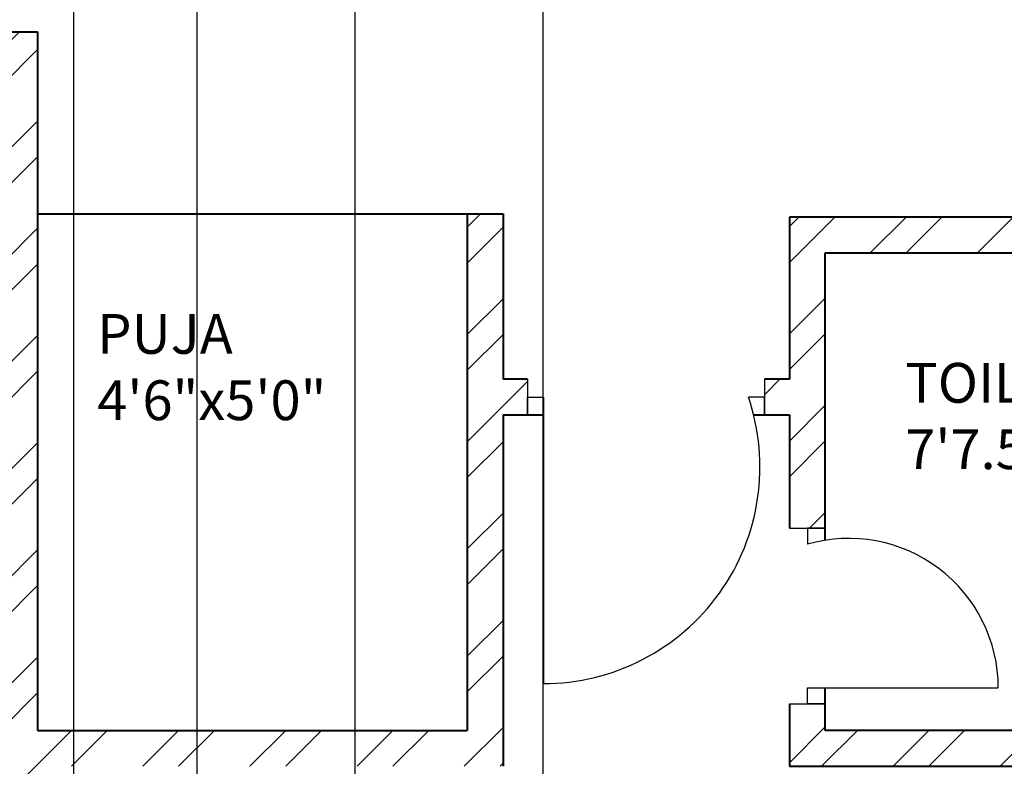
# Model space of a CAD drawing. Units: inches. Extents: x 1601 to 2297, y 1496 to 2631.
# Tile 24 of 57: x 2033 to 2157, y 1793 to 1887. Entities that reach past the tile are written whole.
import ezdxf

# ---------------------------------------------------------------- set-up
doc = ezdxf.new("R2010")
doc.units = ezdxf.units.IN
for name, color, linetype, lineweight in [('A-ANNO-DIMS', 2, 'Continuous', 18), ('A-AREA-IDEN', 7, 'Continuous', 18), ('A-DOOR', 21, 'Continuous', 25), ('A-WALL', 7, 'Continuous', 40), ('A-WALL-PATT', 215, 'Continuous', 13)]:
    doc.layers.add(name, color=color, linetype=linetype, lineweight=lineweight)
doc.styles.get("Standard").update_dxf_attribs({"font": 'arial.ttf'})
doc.dimstyles.get("Standard").update_dxf_attribs({"dimtxt": 0.18, "dimasz": 0.18, "dimexe": 0.18, "dimexo": 0.0625, "dimgap": 0.09, "dimtad": 0, "dimtih": 1, "dimtoh": 1, "dimdec": 4, "dimzin": 0, "dimdsep": 46, "dimtxsty": 'Standard', "dimcen": 0.09, "dimadec": 0, "dimazin": 0, "dimtfac": 1, "dimtdec": 4, "dimtofl": 0, "dimtmove": 0, "dimatfit": 3, "dimfxl": 1, "dimtolj": 1, "dimtzin": 0, "dimarcsym": 0})

# ---------------------------------------------------------------- blocks, each defined once
blk = doc.blocks.new('*D39')
at = {"layer": 'A-ANNO-DIMS', "color": 0, "lineweight": -2, "transparency": 16777216}
for p, q in [((2055.55, 1981.76), (2055.55, 1513.75)), ((2099.05, 1981.76), (2099.05, 1513.75)), ((2055.73, 1513.93), (2076.97, 1513.93)), ((2098.87, 1513.93), (2077.63, 1513.93))]:
    blk.add_line(p, q, dxfattribs=at)
at = {"layer": 'A-ANNO-DIMS', "color": 0, "transparency": 16777216}
for points in [[(2055.73, 1513.96), (2055.73, 1513.9), (2055.55, 1513.93)], [(2098.87, 1513.96), (2098.87, 1513.9), (2099.05, 1513.93)]]:
    blk.add_solid(points, dxfattribs=at)
at = {"layer": 'Defpoints', "color": 0, "transparency": 16777216}
for p in [(2055.55, 1981.83), (2099.05, 1981.83), (2099.05, 1513.93)]:
    blk.add_point(p, dxfattribs=at)
at = {"layer": 'A-ANNO-DIMS', "color": 0, "transparency": 16777216, "insert": (2077.3, 1513.93), "char_height": 0.18, "attachment_point": 5}
blk.add_mtext('\\A1;43.5', dxfattribs=at)
blk = doc.blocks.new('*D41')
at = {"layer": 'A-ANNO-DIMS', "color": 0, "lineweight": -2, "transparency": 16777216}
for p, q in [((2075.4, 2070.14), (2075.4, 1513.75)), ((2040.04, 2066.51), (2040.04, 1513.75)), ((2040.22, 1513.93), (2057.32, 1513.93)), ((2075.22, 1513.93), (2058.11, 1513.93))]:
    blk.add_line(p, q, dxfattribs=at)
at = {"layer": 'A-ANNO-DIMS', "color": 0, "transparency": 16777216}
for points in [[(2040.22, 1513.96), (2040.22, 1513.9), (2040.04, 1513.93)], [(2075.22, 1513.96), (2075.22, 1513.9), (2075.4, 1513.93)]]:
    blk.add_solid(points, dxfattribs=at)
at = {"layer": 'Defpoints', "color": 0, "transparency": 16777216}
for p in [(2075.4, 2070.2), (2040.04, 2066.58), (2075.4, 1513.93)]:
    blk.add_point(p, dxfattribs=at)
at = {"layer": 'A-ANNO-DIMS', "color": 0, "transparency": 16777216, "insert": (2057.72, 1513.93), "char_height": 0.18, "attachment_point": 5}
blk.add_mtext('\\A1;35.36', dxfattribs=at)

msp = doc.modelspace()

# ---------------------------------------------------------------- hatches: boundary and pattern name
at = {"layer": 'A-WALL-PATT'}
h = msp.add_hatch(dxfattribs=at)
h.set_pattern_fill('ANSI32', color=256)
h.paths.add_polyline_path([(1842.0336, 2528.0767), (1842.0336, 2532.3254), (1686.0373, 2532.3254), (1686.0373, 2492.9493), (1695.0373, 2492.9493), (1695.0373, 2523.3254), (1827.0373, 2523.3254), (1827.0373, 2416.8254), (1834.6225, 2416.8254), (1834.6225, 2419.0754), (1834.6225, 2421.3254), (1831.5373, 2421.3254), (1831.5373, 2523.3254), (1842.0336, 2523.3254)])
h.paths.add_polyline_path([(1695.0373, 2432.9493), (1686.0373, 2432.9493), (1686.0373, 2325.989), (1695.0373, 2325.989), (1695.0373, 2347.8254), (1827.0373, 2347.8254), (1827.0373, 2287.8254), (1823.2991, 2287.8254), (1823.2991, 2283.3254), (1847.9422, 2283.3254), (1847.9422, 2285.5754), (1847.9422, 2287.8254), (1831.5373, 2287.8254), (1831.5373, 2347.8254), (1846.9946, 2347.8254), (1846.9946, 2350.0754), (1846.9946, 2352.3254), (1695.0373, 2352.3254)])
h.paths.add_polyline_path([(1807.1169, 1573.5395), (2055.0405, 1573.5395), (2055.0405, 1610.6322), (1807.1169, 1610.6322)], flags=9)
h.paths.add_polyline_path([(1841.1631, 1712.7967), (1870.3957, 1712.7967), (1870.3957, 1731.454), (1841.1631, 1731.454)], flags=9)
h.paths.add_polyline_path([(2144.3862, 1772.185), (2191.0233, 1772.185), (2191.0233, 1790.8423), (2144.3862, 1790.8423)], flags=9)
h.paths.add_polyline_path([(2143.0128, 1827.3312), (2177.9958, 1827.3312), (2177.9958, 1845.9886), (2143.0128, 1845.9886)], flags=9)
h.paths.add_polyline_path([(2041.2439, 1833.5691), (2070.8516, 1833.5691), (2070.8516, 1852.2264), (2041.2439, 1852.2264)], flags=9)
h.paths.add_polyline_path([(2097.2791, 1947.0598), (2134.2061, 1947.0598), (2134.2061, 1965.7171), (2097.2791, 1965.7171)], flags=9)
h.paths.add_polyline_path([(2214.995, 1904.3124), (2214.995, 1942.2899), (2196.3376, 1942.2899), (2196.3376, 1904.3124)], flags=9)
h.paths.add_polyline_path([(2186.6284, 2043.8031), (2219.7935, 2043.8031), (2219.7935, 2062.4605), (2186.6284, 2062.4605)], flags=9)
h.paths.add_polyline_path([(2064.0877, 2031.616), (2097.4949, 2031.616), (2097.4949, 2050.2734), (2064.0877, 2050.2734)], flags=9)
h.paths.add_polyline_path([(1973.1349, 1986.0688), (2008.4009, 1986.0688), (2008.4009, 2004.7261), (1973.1349, 2004.7261)], flags=9)
h.paths.add_polyline_path([(1976.3676, 2106.9635), (2005.7469, 2106.9635), (2005.7469, 2125.6209), (1976.3676, 2125.6209)], flags=9)
h.paths.add_polyline_path([(1991.7852, 2180.4863), (2027.0513, 2180.4863), (2027.0513, 2199.1437), (1991.7852, 2199.1437)], flags=9)
h.paths.add_polyline_path([(2106.1801, 2187.9359), (2152.2101, 2187.9359), (2152.2101, 2206.5932), (2106.1801, 2206.5932)], flags=9)
h.paths.add_polyline_path([(2148.6686, 2262.2542), (2182.318, 2262.2542), (2182.318, 2280.9115), (2148.6686, 2280.9115)], flags=9)
h.paths.add_polyline_path([(2041.6327, 2252.8147), (2071.2405, 2252.8147), (2071.2405, 2271.4721), (2041.6327, 2271.4721)], flags=9)
h.paths.add_polyline_path([(2063.9734, 2375.4265), (2100.9004, 2375.4265), (2100.9004, 2394.0839), (2063.9734, 2394.0839)], flags=9)
h.paths.add_polyline_path([(2216.4955, 2330.9748), (2216.4955, 2370.2654), (2197.8381, 2370.2654), (2197.8381, 2330.9748)], flags=9)
h.paths.add_polyline_path([(2179.1416, 2485.8687), (2212.3067, 2485.8687), (2212.3067, 2504.5261), (2179.1416, 2504.5261)], flags=9)
h.paths.add_polyline_path([(2078.7442, 2471.1516), (2112.1514, 2471.1516), (2112.1514, 2489.809), (2078.7442, 2489.809)], flags=9)
h.paths.add_polyline_path([(1915.9631, 2329.4668), (1952.8902, 2329.4668), (1952.8902, 2348.1241), (1915.9631, 2348.1241)], flags=9)
h.paths.add_polyline_path([(1904.3189, 2499.6709), (1940.4512, 2499.6709), (1940.4512, 2518.3282), (1904.3189, 2518.3282)], flags=9)
h.paths.add_polyline_path([(1892.3665, 2100.4595), (1925.6374, 2100.4595), (1925.6374, 2119.1169), (1892.3665, 2119.1169)], flags=9)
h.paths.add_polyline_path([(1909.2984, 1805.9631), (1946.2254, 1805.9631), (1946.2254, 1824.6205), (1909.2984, 1824.6205)], flags=9)
h.paths.add_polyline_path([(1934.6056, 1658.616), (1970.738, 1658.616), (1970.738, 1677.2733), (1934.6056, 1677.2733)], flags=9)
h.paths.add_polyline_path([(1711.2052, 1789.8902), (1750.0456, 1789.8902), (1750.0456, 1808.5476), (1711.2052, 1808.5476)], flags=9)
h.paths.add_polyline_path([(1742.7874, 1854.6743), (1771.9449, 1854.6743), (1771.9449, 1873.3317), (1742.7874, 1873.3317)], flags=9)
h.paths.add_polyline_path([(1807.3592, 1997.7912), (1850.1116, 1997.7912), (1850.1116, 2016.4486), (1807.3592, 2016.4486)], flags=9)
h.paths.add_polyline_path([(1717.4579, 2237.7844), (1760.2103, 2237.7844), (1760.2103, 2256.4417), (1717.4579, 2256.4417)], flags=9)
h.paths.add_polyline_path([(1780.9285, 2324.0623), (1810.086, 2324.0623), (1810.086, 2342.7197), (1780.9285, 2342.7197)], flags=25)
h.paths.add_polyline_path([(1837.696, 2449.2024), (1866.9286, 2449.2024), (1866.9286, 2467.8598), (1837.696, 2467.8598)], flags=9)
h.paths.add_polyline_path([(1712.7752, 2484.9404), (1751.6156, 2484.9404), (1751.6156, 2503.5977), (1712.7752, 2503.5977)], flags=25)
h = msp.add_hatch(dxfattribs=at)
h.set_pattern_fill('ANSI32', color=256)
h.paths.add_polyline_path([(1973.9371, 2211.3254), (1893.0373, 2211.3254), (1893.0373, 2287.8254), (1884.6167, 2287.8254), (1884.6167, 2285.5754), (1884.6167, 2283.3254), (1888.5373, 2283.3254), (1888.5373, 2145.3254), (1695.0373, 2145.3254), (1695.0373, 2173.8724), (1690.5373, 2173.8724), (1686.0373, 2173.8724), (1686.0373, 2136.3254), (1722.5687, 2136.3254), (1722.5687, 2117.4352), (1731.5687, 2117.4352), (1731.5687, 2136.3254), (1893.0373, 2136.3254), (1893.0373, 2202.3254), (1959.0373, 2202.3254), (1959.0373, 2182.1303), (1968.0373, 2182.1303), (1968.0373, 2202.3254), (1973.9371, 2202.3254)])
h.paths.add_polyline_path([(2094.0373, 2274.6364), (2096.4294, 2274.6364), (2096.4294, 2276.8864), (2096.4294, 2279.1364), (2094.0373, 2279.1364), (2094.0373, 2290.8254), (2094.0373, 2295.3254), (2089.5373, 2295.3254), (2089.5373, 2230.8254), (2035.5373, 2230.8254), (2035.5373, 2299.8254), (2031.0373, 2299.8254), (2031.0373, 2211.3254), (2023.0065, 2211.3254), (2023.0065, 2202.3254), (2031.0373, 2202.3254), (2031.0373, 2140.8254), (1968.0373, 2140.8254), (1968.0373, 2145.9106), (1963.5373, 2145.9106), (1959.0373, 2145.9106), (1959.0373, 2116.839), (1963.5373, 2116.839), (1968.0373, 2116.839), (1968.0373, 2131.8254), (2031.0373, 2131.8254), (2031.0373, 2094.3254), (2031.0373, 2085.3254), (2031.0373, 2056.8254), (1968.0373, 2056.8254), (1968.0373, 2070.4947), (1963.5373, 2070.4947), (1959.0373, 2070.4947), (1959.0373, 2040.3029), (1968.0373, 2040.3029), (1968.0373, 2047.8254), (2031.0373, 2047.8254), (2031.0373, 1983.3254), (2031.0373, 1978.8254), (2021.1979, 1978.8254), (2021.1979, 1974.3254), (2031.0373, 1974.3254), (2031.0373, 1954.3528), (2035.5373, 1954.3528), (2035.5373, 1974.3254), (2035.5373, 1981.8254), (2055.5513, 1981.8254), (2055.5513, 1986.3254), (2035.5373, 1986.3254), (2035.5373, 2047.8254), (2040.0373, 2047.8254), (2040.0373, 2085.3254), (2040.0373, 2094.3254), (2040.0373, 2140.8254), (2035.5373, 2140.8254), (2035.5373, 2226.3254), (2089.5373, 2226.3254), (2094.0373, 2226.3254)])
h.paths.add_polyline_path([(2226.0373, 2230.8254), (2134.5373, 2230.8254), (2134.5373, 2233.5437), (2130.0373, 2233.5437), (2130.0373, 2226.3254), (2134.5373, 2226.3254), (2226.0373, 2226.3254)])
h.paths.add_polyline_path([(1807.1169, 1573.5395), (2055.0405, 1573.5395), (2055.0405, 1610.6322), (1807.1169, 1610.6322)], flags=9)
h.paths.add_polyline_path([(1841.1631, 1712.7967), (1870.3957, 1712.7967), (1870.3957, 1731.454), (1841.1631, 1731.454)], flags=9)
h.paths.add_polyline_path([(2144.3862, 1772.185), (2191.0233, 1772.185), (2191.0233, 1790.8423), (2144.3862, 1790.8423)], flags=9)
h.paths.add_polyline_path([(2143.0128, 1827.3312), (2177.9958, 1827.3312), (2177.9958, 1845.9886), (2143.0128, 1845.9886)], flags=9)
h.paths.add_polyline_path([(2041.2439, 1833.5691), (2070.8516, 1833.5691), (2070.8516, 1852.2264), (2041.2439, 1852.2264)], flags=9)
h.paths.add_polyline_path([(2097.2791, 1947.0598), (2134.2061, 1947.0598), (2134.2061, 1965.7171), (2097.2791, 1965.7171)], flags=9)
h.paths.add_polyline_path([(2214.995, 1904.3124), (2214.995, 1942.2899), (2196.3376, 1942.2899), (2196.3376, 1904.3124)], flags=9)
h.paths.add_polyline_path([(2186.6284, 2043.8031), (2219.7935, 2043.8031), (2219.7935, 2062.4605), (2186.6284, 2062.4605)], flags=9)
h.paths.add_polyline_path([(2064.0877, 2031.616), (2097.4949, 2031.616), (2097.4949, 2050.2734), (2064.0877, 2050.2734)], flags=9)
h.paths.add_polyline_path([(1973.1349, 1986.0688), (2008.4009, 1986.0688), (2008.4009, 2004.7261), (1973.1349, 2004.7261)], flags=25)
h.paths.add_polyline_path([(1976.3676, 2106.9635), (2005.7469, 2106.9635), (2005.7469, 2125.6209), (1976.3676, 2125.6209)], flags=25)
h.paths.add_polyline_path([(1991.7852, 2180.4863), (2027.0513, 2180.4863), (2027.0513, 2199.1437), (1991.7852, 2199.1437)], flags=25)
h.paths.add_polyline_path([(2106.1801, 2187.9359), (2152.2101, 2187.9359), (2152.2101, 2206.5932), (2106.1801, 2206.5932)], flags=9)
h.paths.add_polyline_path([(2148.6686, 2262.2542), (2182.318, 2262.2542), (2182.318, 2280.9115), (2148.6686, 2280.9115)], flags=9)
h.paths.add_polyline_path([(2041.6327, 2252.8147), (2071.2405, 2252.8147), (2071.2405, 2271.4721), (2041.6327, 2271.4721)], flags=25)
h.paths.add_polyline_path([(2063.9734, 2375.4265), (2100.9004, 2375.4265), (2100.9004, 2394.0839), (2063.9734, 2394.0839)], flags=9)
h.paths.add_polyline_path([(2216.4955, 2330.9748), (2216.4955, 2370.2654), (2197.8381, 2370.2654), (2197.8381, 2330.9748)], flags=9)
h.paths.add_polyline_path([(2179.1416, 2485.8687), (2212.3067, 2485.8687), (2212.3067, 2504.5261), (2179.1416, 2504.5261)], flags=9)
h.paths.add_polyline_path([(2078.7442, 2471.1516), (2112.1514, 2471.1516), (2112.1514, 2489.809), (2078.7442, 2489.809)], flags=9)
h.paths.add_polyline_path([(1915.9631, 2329.4668), (1952.8902, 2329.4668), (1952.8902, 2348.1241), (1915.9631, 2348.1241)], flags=9)
h.paths.add_polyline_path([(1904.3189, 2499.6709), (1940.4512, 2499.6709), (1940.4512, 2518.3282), (1904.3189, 2518.3282)], flags=9)
h.paths.add_polyline_path([(1892.3665, 2100.4595), (1925.6374, 2100.4595), (1925.6374, 2119.1169), (1892.3665, 2119.1169)], flags=9)
h.paths.add_polyline_path([(1909.2984, 1805.9631), (1946.2254, 1805.9631), (1946.2254, 1824.6205), (1909.2984, 1824.6205)], flags=9)
h.paths.add_polyline_path([(1934.6056, 1658.616), (1970.738, 1658.616), (1970.738, 1677.2733), (1934.6056, 1677.2733)], flags=9)
h.paths.add_polyline_path([(1711.2052, 1789.8902), (1750.0456, 1789.8902), (1750.0456, 1808.5476), (1711.2052, 1808.5476)], flags=9)
h.paths.add_polyline_path([(1742.7874, 1854.6743), (1771.9449, 1854.6743), (1771.9449, 1873.3317), (1742.7874, 1873.3317)], flags=9)
h.paths.add_polyline_path([(1807.3592, 1997.7912), (1850.1116, 1997.7912), (1850.1116, 2016.4486), (1807.3592, 2016.4486)], flags=9)
h.paths.add_polyline_path([(1717.4579, 2237.7844), (1760.2103, 2237.7844), (1760.2103, 2256.4417), (1717.4579, 2256.4417)], flags=25)
h.paths.add_polyline_path([(1780.9285, 2324.0623), (1810.086, 2324.0623), (1810.086, 2342.7197), (1780.9285, 2342.7197)], flags=9)
h.paths.add_polyline_path([(1837.696, 2449.2024), (1866.9286, 2449.2024), (1866.9286, 2467.8598), (1837.696, 2467.8598)], flags=9)
h.paths.add_polyline_path([(1712.7752, 2484.9404), (1751.6156, 2484.9404), (1751.6156, 2503.5977), (1712.7752, 2503.5977)], flags=9)
h = msp.add_hatch(dxfattribs=at)
h.set_pattern_fill('ANSI32', color=256)
h.paths.add_polyline_path([(2230.5373, 1861.8254), (2182.5373, 1861.8254), (2182.5373, 1885.3637), (2178.0373, 1885.3637), (2178.0373, 1861.8254), (2166.0373, 1861.8254), (2134.5373, 1861.8254), (2130.0373, 1861.8254), (2130.0373, 1841.4682), (2126.8833, 1841.4682), (2126.8833, 1836.9682), (2130.0373, 1836.9682), (2130.0373, 1822.7302), (2134.5373, 1822.7302), (2134.5373, 1857.3254), (2166.0373, 1857.3254), (2226.0373, 1857.3254), (2226.0373, 1846.1155), (2230.5373, 1846.1155)])
h.paths.add_polyline_path([(2226.0373, 1797.3254), (2134.5373, 1797.3254), (2134.5373, 1800.6636), (2132.2873, 1800.6636), (2130.0373, 1800.6636), (2130.0373, 1797.3254), (2130.0373, 1792.8254), (2167.7264, 1792.8254), (2226.0373, 1792.8254)])
h.paths.add_polyline_path([(2230.5373, 1822.1155), (2226.0373, 1822.1155), (2226.0373, 1760.8563), (2230.5373, 1760.8563)])
h.paths.add_polyline_path([(2230.5373, 1700.8563), (2226.0373, 1700.8563), (2226.0373, 1644.3254), (2140.2517, 1644.3254), (2140.2517, 1635.3254), (2230.5373, 1635.3254)])
h.paths.add_polyline_path([(2080.2517, 1639.8254), (2080.2517, 1644.3254), (2035.5373, 1644.3254), (2035.5373, 1792.8254), (2094.0373, 1792.8254), (2094.0373, 1797.3254), (2094.0373, 1836.9682), (2097.1057, 1836.9682), (2097.1057, 1839.2182), (2097.1057, 1841.4682), (2094.0373, 1841.4682), (2094.0373, 1862.2276), (2089.5373, 1862.2276), (2089.5373, 1797.3254), (2035.5373, 1797.3254), (2035.5373, 1857.3254), (2035.5373, 1885.0916), (2031.0373, 1885.0916), (2031.0373, 1710.3254), (2012.329, 1710.3254), (2012.329, 1701.3254), (2031.0373, 1701.3254), (2031.0373, 1644.3254), (2031.0373, 1635.3254), (2080.2517, 1635.3254)])
h.paths.add_polyline_path([(1836.0373, 1653.2033), (1842.6171, 1653.2033), (1842.6171, 1657.7033), (1842.6171, 1662.2033), (1831.5373, 1662.2033), (1831.5373, 1764.2033), (1835.3881, 1764.2033), (1835.3881, 1766.4533), (1835.3881, 1768.7033), (1831.5373, 1768.7033), (1827.0373, 1768.7033), (1827.0373, 1662.2033), (1827.0373, 1635.3254), (1836.0373, 1635.3254)])
h.paths.add_polyline_path([(1893.0373, 1701.3254), (1907.193, 1701.3254), (1907.193, 1705.8254), (1907.193, 1710.3254), (1893.0373, 1710.3254), (1893.0373, 1819.8254), (1882.6444, 1819.8254), (1882.6444, 1817.5754), (1882.6444, 1815.3254), (1888.5373, 1815.3254), (1888.5373, 1662.2033), (1884.0373, 1662.2033), (1866.6171, 1662.2033), (1866.6171, 1653.2033), (1882.391, 1653.2033), (1884.0373, 1653.2033), (1884.0373, 1635.3254), (1893.0373, 1635.3254)])
h.paths.add_polyline_path([(1739.3335, 1639.8254), (1739.3335, 1644.3254), (1695.0373, 1644.3254), (1695.0373, 1702.0135), (1690.5373, 1702.0135), (1686.0373, 1702.0135), (1686.0373, 1635.3254), (1739.3335, 1635.3254)])
h.paths.add_polyline_path([(1827.0373, 1644.3254), (1799.3335, 1644.3254), (1799.3335, 1635.3254), (1827.0373, 1635.3254)])
h.paths.add_polyline_path([(1695.0373, 1815.3254), (1849.2759, 1815.3254), (1849.2759, 1819.8254), (1807.5373, 1819.8254), (1807.5373, 1879.8254), (1851.1533, 1879.8254), (1851.1533, 1882.0754), (1851.1533, 1884.3254), (1799.3405, 1884.3254), (1799.3405, 1882.0754), (1799.3405, 1879.8254), (1803.0373, 1879.8254), (1803.0373, 1819.8254), (1695.0373, 1819.8254), (1695.0373, 1835.0458), (1690.5373, 1835.0458), (1686.0373, 1835.0458), (1686.0373, 1766.1753), (1695.0373, 1766.1753)])
h.paths.add_polyline_path([(1775.8157, 1884.3254), (1695.0373, 1884.3254), (1695.0373, 1912.9526), (1690.5373, 1912.9526), (1686.0373, 1912.9526), (1686.0373, 1859.0458), (1695.0373, 1859.0458), (1695.0373, 1879.8254), (1775.8157, 1879.8254)])
h.paths.add_polyline_path([(1893.0373, 2031.3254), (1731.5687, 2031.3254), (1731.5687, 2057.4352), (1722.5687, 2057.4352), (1722.5687, 2031.3254), (1686.0373, 2031.3254), (1686.0373, 1972.9526), (1695.0373, 1972.9526), (1695.0373, 2022.3254), (1888.5373, 2022.3254), (1888.5373, 1884.3254), (1883.4996, 1884.3254), (1883.4996, 1879.8254), (1893.0373, 1879.8254), (1893.0373, 1974.3254), (1976.6199, 1974.3254), (1976.6199, 1978.8254), (1968.0373, 1978.8254), (1968.0373, 1983.3254), (1968.0373, 2008.4756), (1963.5373, 2008.4756), (1959.0373, 2008.4756), (1959.0373, 1983.3254), (1893.0373, 1983.3254)])
h.paths.add_polyline_path([(2230.5373, 2140.4745), (2226.0373, 2140.4745), (2226.0373, 2094.3254), (2040.0373, 2094.3254), (2040.0373, 2085.3254), (2178.0373, 2085.3254), (2178.0373, 2065.6965), (2182.5373, 2065.6965), (2182.5373, 2085.3254), (2226.0373, 2085.3254), (2226.0373, 1986.3254), (2211.2679, 1986.3254), (2211.2679, 1981.8254), (2230.5373, 1981.8254)])
h.paths.add_polyline_path([(2187.6292, 1986.3254), (2182.5373, 1986.3254), (2182.5373, 2029.6965), (2178.0373, 2029.6965), (2178.0373, 1986.3254), (2099.05, 1986.3254), (2099.05, 1981.8254), (2178.0373, 1981.8254), (2178.0373, 1969.3637), (2182.5373, 1969.3637), (2182.5373, 1981.8254), (2187.6292, 1981.8254), (2187.6292, 1984.0754)])
h.paths.add_polyline_path([(1807.1169, 1573.5395), (2055.0405, 1573.5395), (2055.0405, 1610.6322), (1807.1169, 1610.6322)], flags=9)
h.paths.add_polyline_path([(1841.1631, 1712.7967), (1870.3957, 1712.7967), (1870.3957, 1731.454), (1841.1631, 1731.454)], flags=9)
h.paths.add_polyline_path([(2144.3862, 1772.185), (2191.0233, 1772.185), (2191.0233, 1790.8423), (2144.3862, 1790.8423)], flags=9)
h.paths.add_polyline_path([(2143.0128, 1827.3312), (2177.9958, 1827.3312), (2177.9958, 1845.9886), (2143.0128, 1845.9886)], flags=25)
h.paths.add_polyline_path([(2041.2439, 1833.5691), (2070.8516, 1833.5691), (2070.8516, 1852.2264), (2041.2439, 1852.2264)], flags=25)
h.paths.add_polyline_path([(2097.2791, 1947.0598), (2134.2061, 1947.0598), (2134.2061, 1965.7171), (2097.2791, 1965.7171)], flags=9)
h.paths.add_polyline_path([(2214.995, 1904.3124), (2214.995, 1942.2899), (2196.3376, 1942.2899), (2196.3376, 1904.3124)], flags=9)
h.paths.add_polyline_path([(2186.6284, 2043.8031), (2219.7935, 2043.8031), (2219.7935, 2062.4605), (2186.6284, 2062.4605)], flags=25)
h.paths.add_polyline_path([(2064.0877, 2031.616), (2097.4949, 2031.616), (2097.4949, 2050.2734), (2064.0877, 2050.2734)], flags=25)
h.paths.add_polyline_path([(1973.1349, 1986.0688), (2008.4009, 1986.0688), (2008.4009, 2004.7261), (1973.1349, 2004.7261)], flags=9)
h.paths.add_polyline_path([(1976.3676, 2106.9635), (2005.7469, 2106.9635), (2005.7469, 2125.6209), (1976.3676, 2125.6209)], flags=9)
h.paths.add_polyline_path([(1991.7852, 2180.4863), (2027.0513, 2180.4863), (2027.0513, 2199.1437), (1991.7852, 2199.1437)], flags=9)
h.paths.add_polyline_path([(2106.1801, 2187.9359), (2152.2101, 2187.9359), (2152.2101, 2206.5932), (2106.1801, 2206.5932)], flags=9)
h.paths.add_polyline_path([(2148.6686, 2262.2542), (2182.318, 2262.2542), (2182.318, 2280.9115), (2148.6686, 2280.9115)], flags=9)
h.paths.add_polyline_path([(2041.6327, 2252.8147), (2071.2405, 2252.8147), (2071.2405, 2271.4721), (2041.6327, 2271.4721)], flags=9)
h.paths.add_polyline_path([(2063.9734, 2375.4265), (2100.9004, 2375.4265), (2100.9004, 2394.0839), (2063.9734, 2394.0839)], flags=9)
h.paths.add_polyline_path([(2216.4955, 2330.9748), (2216.4955, 2370.2654), (2197.8381, 2370.2654), (2197.8381, 2330.9748)], flags=9)
h.paths.add_polyline_path([(2179.1416, 2485.8687), (2212.3067, 2485.8687), (2212.3067, 2504.5261), (2179.1416, 2504.5261)], flags=9)
h.paths.add_polyline_path([(2078.7442, 2471.1516), (2112.1514, 2471.1516), (2112.1514, 2489.809), (2078.7442, 2489.809)], flags=9)
h.paths.add_polyline_path([(1915.9631, 2329.4668), (1952.8902, 2329.4668), (1952.8902, 2348.1241), (1915.9631, 2348.1241)], flags=9)
h.paths.add_polyline_path([(1904.3189, 2499.6709), (1940.4512, 2499.6709), (1940.4512, 2518.3282), (1904.3189, 2518.3282)], flags=9)
h.paths.add_polyline_path([(1892.3665, 2100.4595), (1925.6374, 2100.4595), (1925.6374, 2119.1169), (1892.3665, 2119.1169)], flags=9)
h.paths.add_polyline_path([(1909.2984, 1805.9631), (1946.2254, 1805.9631), (1946.2254, 1824.6205), (1909.2984, 1824.6205)], flags=9)
h.paths.add_polyline_path([(1934.6056, 1658.616), (1970.738, 1658.616), (1970.738, 1677.2733), (1934.6056, 1677.2733)], flags=9)
h.paths.add_polyline_path([(1711.2052, 1789.8902), (1750.0456, 1789.8902), (1750.0456, 1808.5476), (1711.2052, 1808.5476)], flags=25)
h.paths.add_polyline_path([(1742.7874, 1854.6743), (1771.9449, 1854.6743), (1771.9449, 1873.3317), (1742.7874, 1873.3317)], flags=25)
h.paths.add_polyline_path([(1807.3592, 1997.7912), (1850.1116, 1997.7912), (1850.1116, 2016.4486), (1807.3592, 2016.4486)], flags=25)
h.paths.add_polyline_path([(1717.4579, 2237.7844), (1760.2103, 2237.7844), (1760.2103, 2256.4417), (1717.4579, 2256.4417)], flags=9)
h.paths.add_polyline_path([(1780.9285, 2324.0623), (1810.086, 2324.0623), (1810.086, 2342.7197), (1780.9285, 2342.7197)], flags=9)
h.paths.add_polyline_path([(1837.696, 2449.2024), (1866.9286, 2449.2024), (1866.9286, 2467.8598), (1837.696, 2467.8598)], flags=9)
h.paths.add_polyline_path([(1712.7752, 2484.9404), (1751.6156, 2484.9404), (1751.6156, 2503.5977), (1712.7752, 2503.5977)], flags=9)

# ---------------------------------------------------------------- linework, layer by layer
at = {"layer": 'A-DOOR'}
for p, q in [((2097.1057, 1841.4682), (2097.1057, 1836.9682)), ((2126.8833, 1841.4682), (2126.8833, 1836.9682)), ((2097.1057, 1836.9682), (2097.1057, 1839.2182)), ((2097.1057, 1839.2182), (2099.1057, 1839.2182)), ((2099.1057, 1839.2182), (2099.1057, 1803.2182)), ((2126.8833, 1839.2182), (2124.8833, 1839.2182)), ((2126.8833, 1836.9682), (2126.8833, 1839.2182)), ((2130.0373, 1822.7302), (2134.5373, 1822.7302)), ((2134.5373, 1822.7302), (2132.2873, 1822.7302)), ((2132.2873, 1822.7302), (2132.2873, 1820.7302)), ((2132.2873, 1800.6636), (2132.2873, 1802.6636)), ((2132.2873, 1802.6636), (2156.2873, 1802.6636)), ((2130.0373, 1800.6636), (2134.5373, 1800.6636)), ((2134.5373, 1800.6636), (2132.2873, 1800.6636))]:
    msp.add_line(p, q, dxfattribs=at)
for centre, radius, start, end in [((2099.1057, 1830.4471), 27.2289, 270, 18.791338), ((2137.4872, 1802.6636), 18.8001, 360, 106.056837)]:
    msp.add_arc(centre, radius, start, end, dxfattribs=at)
at = {"layer": 'A-WALL'}
for p, q in [((2031.0373, 1885.0916), (2035.5373, 1885.0916)), ((2035.5373, 1885.0916), (2035.5373, 1797.3254)), ((2035.5373, 1862.2276), (2089.5373, 1862.2276)), ((2089.5373, 1862.2276), (2089.5373, 1797.3254)), ((2089.5373, 1862.2276), (2094.0373, 1862.2276)), ((2094.0373, 1862.2276), (2094.0373, 1841.4682)), ((2134.5373, 1861.8254), (2130.0373, 1861.8254)), ((2130.0373, 1861.8254), (2130.0373, 1841.4682)), ((2166.0373, 1861.8254), (2134.5373, 1861.8254)), ((2035.5373, 1857.3254), (2035.5373, 1797.3254)), ((2134.5373, 1857.3254), (2166.0373, 1857.3254)), ((2134.5373, 1821.2308), (2134.5373, 1857.3254)), ((2097.1057, 1841.4682), (2094.0373, 1841.4682)), ((2130.0373, 1841.4682), (2126.8833, 1841.4682)), ((2094.0373, 1836.9682), (2099.1057, 1836.9682)), ((2094.0373, 1836.9682), (2094.0373, 1797.3254)), ((2125.5422, 1836.9682), (2130.0373, 1836.9682)), ((2130.0373, 1836.9682), (2130.0373, 1822.7302)), ((2035.5373, 1802.2276), (2035.5373, 1797.7276)), ((2134.5373, 1797.3254), (2134.5373, 1802.6636)), ((2130.0373, 1800.6636), (2130.0373, 1797.3254)), ((2035.5373, 1797.3254), (2089.5373, 1797.3254)), ((2094.0373, 1797.3254), (2094.0373, 1792.8254)), ((2130.0373, 1797.3254), (2130.0373, 1792.8254)), ((2226.0373, 1797.3254), (2134.5373, 1797.3254)), ((2130.0373, 1792.8254), (2167.7264, 1792.8254))]:
    msp.add_line(p, q, dxfattribs=at)

# ---------------------------------------------------------------- texts
at = {"layer": 'A-AREA-IDEN', "char_height": 5, "attachment_point": 1}
for s, width, insert in [('PUJA\\P4\'6"x5\'0"', 38.802263, (2043.0327, 1849.6531)), ('TOILET\\P7\'7.5"x5\'0"', 77.548495, (2144.5937, 1843.5039))]:
    msp.add_mtext_dynamic_manual_height_columns(s, width=width, gutter_width=12.5, heights=[0], dxfattribs=dict(at, insert=insert))

# ---------------------------------------------------------------- dimensions: what is measured, and where the dimension line sits
at = {"layer": 'A-ANNO-DIMS'}
for base, p1, p2, override, picture, middle in [((2075.3977, 1513.9279), (2040.0373, 2066.5754), (2075.3977, 2070.1988), {"dimdec": 2, "dimlfac": 1, "dimrnd": 0, "dimzin": 0, "dimdsep": 46, "dimlunit": 2}, '*D41', (2057.7175, 1513.9279)), ((2099.05, 1513.9279), (2055.5513, 1981.8254), (2099.05, 1981.8254), {"dimdec": 1, "dimlfac": 1, "dimrnd": 0, "dimzin": 0, "dimdsep": 46, "dimlunit": 2}, '*D39', (2077.3006, 1513.9279))]:
    dim = msp.add_linear_dim(base=base, p1=p1, p2=p2, dimstyle='Standard', override=override, dxfattribs=at)
    dim.commit()
    dim.dimension.update_dxf_attribs({"geometry": picture, "text_midpoint": middle})

doc.saveas('drawing.dxf')
